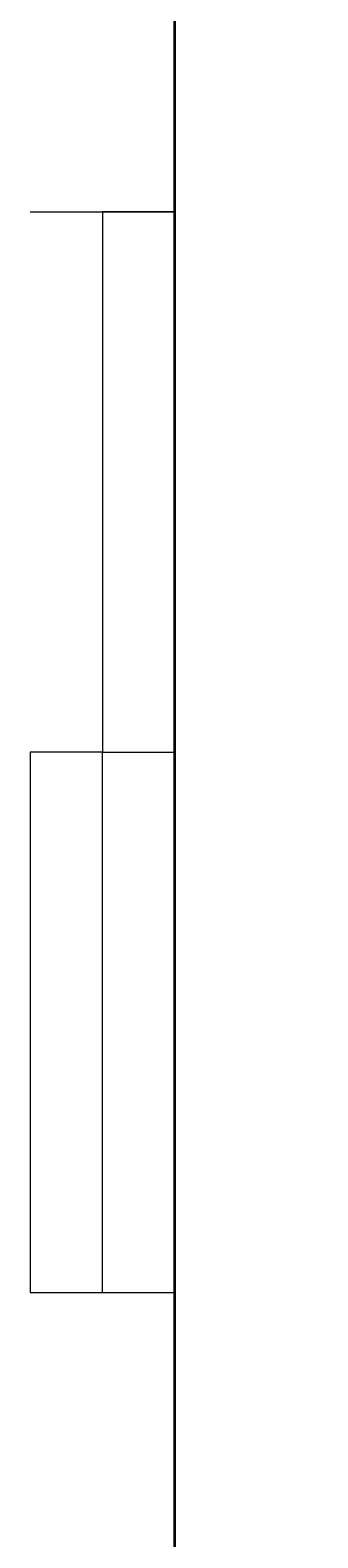
# Model space of a CAD drawing. Units: inches. Extents: x -61 to 1599, y -1316 to 257.
# Tile 101 of 204: x 114 to 126, y -131 to -68. Entities that reach past the tile are written whole.
import ezdxf

# ---------------------------------------------------------------- set-up
doc = ezdxf.new("R2010")
doc.units = ezdxf.units.IN
doc.header["$MEASUREMENT"] = 0
for name, color, linetype, lineweight in [('A-ANNO-DIMS', 2, 'Continuous', 18), ('WALLS', 4, 'Continuous', 35), ('WINDOWS', 220, 'Continuous', 18)]:
    doc.layers.add(name, color=color, linetype=linetype, lineweight=lineweight)
doc.styles.get("Standard").update_dxf_attribs({"font": 'arial.ttf'})
doc.dimstyles.get("Standard").update_dxf_attribs({"dimtxt": 0.18, "dimasz": 0.18, "dimexe": 0.18, "dimexo": 0.0625, "dimgap": 0.09, "dimtad": 0, "dimtih": 1, "dimtoh": 1, "dimdec": 0, "dimzin": 0, "dimdsep": 46, "dimlunit": 3, "dimtxsty": 'Standard', "dimcen": 0.09, "dimadec": 0, "dimazin": 0, "dimtfac": 1, "dimtdec": 0, "dimtofl": 0, "dimtmove": 0, "dimatfit": 3, "dimfxl": 1, "dimtolj": 1, "dimtzin": 0, "dimarcsym": 0})

# ---------------------------------------------------------------- blocks, each defined once
blk = doc.blocks.new('WIN-45IN')
for p, q in [((0, 44.83), (6, 44.83)), ((0, 0), (6, 0))]:
    blk.add_line(p, q)
for points in [[(6, 44.83), (3, 44.83), (3, 22.415), (6, 22.415)], [(3, 22.415), (0, 22.415), (0, 0), (3, 0)]]:
    blk.add_lwpolyline(points, close=True)
blk = doc.blocks.new('*D687')
at = {"layer": 'A-ANNO-DIMS', "color": 0, "lineweight": -2, "transparency": 16777216}
for p, q in [((289.418, 181.677), (-61.077, 181.677)), ((-60.897, 181.497), (-60.897, -528.952)), ((-60.897, -1239.765), (-60.897, -529.316)), ((319.64, -1239.945), (-61.077, -1239.945))]:
    blk.add_line(p, q, dxfattribs=at)
at = {"layer": 'A-ANNO-DIMS', "color": 0, "transparency": 16777216}
for points in [[(-60.927, 181.497), (-60.867, 181.497), (-60.897, 181.677)], [(-60.927, -1239.765), (-60.867, -1239.765), (-60.897, -1239.945)]]:
    blk.add_solid(points, dxfattribs=at)
at = {"layer": 'DEFPOINTS', "color": 0, "transparency": 16777216}
for p in [(289.481, 181.677), (-60.897, -1239.945), (319.703, -1239.945)]:
    blk.add_point(p, dxfattribs=at)
at = {"layer": 'A-ANNO-DIMS', "color": 0, "transparency": 16777216, "insert": (-60.897, -529.134), "char_height": 0.18, "attachment_point": 5}
blk.add_mtext('\\A1;1421.6', dxfattribs=at)
blk = doc.blocks.new('*D700')
at = {"layer": 'A-ANNO-DIMS', "color": 0, "lineweight": -2, "transparency": 16777216}
for p, q in [((14.703, -616.882), (14.703, 257.457)), ((14.883, 257.277), (96.772, 257.277)), ((179.572, 257.277), (97.683, 257.277)), ((179.752, -616.882), (179.752, 257.457))]:
    blk.add_line(p, q, dxfattribs=at)
at = {"layer": 'A-ANNO-DIMS', "color": 0, "transparency": 16777216}
for points in [[(14.883, 257.307), (14.883, 257.247), (14.703, 257.277)], [(179.572, 257.307), (179.572, 257.247), (179.752, 257.277)]]:
    blk.add_solid(points, dxfattribs=at)
at = {"layer": 'DEFPOINTS', "color": 0, "transparency": 16777216}
for p in [(179.752, 257.277), (14.703, -616.945), (179.752, -616.945)]:
    blk.add_point(p, dxfattribs=at)
at = {"layer": 'A-ANNO-DIMS', "color": 0, "transparency": 16777216, "insert": (97.227, 257.277), "char_height": 0.18, "attachment_point": 5}
blk.add_mtext('\\A1;165.05', dxfattribs=at)

msp = doc.modelspace()

# ---------------------------------------------------------------- linework, layer by layer
at = {"layer": 'WALLS'}
msp.add_line((119.7028, -169.3229), (119.7028, -13.3229), dxfattribs=at)

# ---------------------------------------------------------------- block references
at = {"layer": 'WINDOWS'}
msp.add_blockref('WIN-45IN', (113.703, -120.498), dxfattribs=at)

# ---------------------------------------------------------------- dimensions: what is measured, and where the dimension line sits
at = {"layer": 'A-ANNO-DIMS'}
dim = msp.add_linear_dim(base=(179.7521, 257.2771), p1=(14.7028, -616.9446), p2=(179.7521, -616.9446), dimstyle='Standard', override={"dimdec": 2, "dimlfac": 1, "dimrnd": 0, "dimzin": 0, "dimdsep": 46, "dimlunit": 2}, dxfattribs=at)
dim.commit()
dim.dimension.update_dxf_attribs({"geometry": '*D700', "text_midpoint": (97.2274, 257.2771)})
dim = msp.add_linear_dim(base=(-60.8972, -1239.9446), p1=(289.4807, 181.6771), p2=(319.7028, -1239.9446), angle=90, dimstyle='Standard', override={"dimdec": 1, "dimlfac": 1, "dimrnd": 0, "dimzin": 0, "dimdsep": 46, "dimlunit": 2}, dxfattribs=at)
dim.commit()
dim.dimension.update_dxf_attribs({"geometry": '*D687', "text_midpoint": (-60.8972, -529.1337)})

doc.saveas('drawing.dxf')
